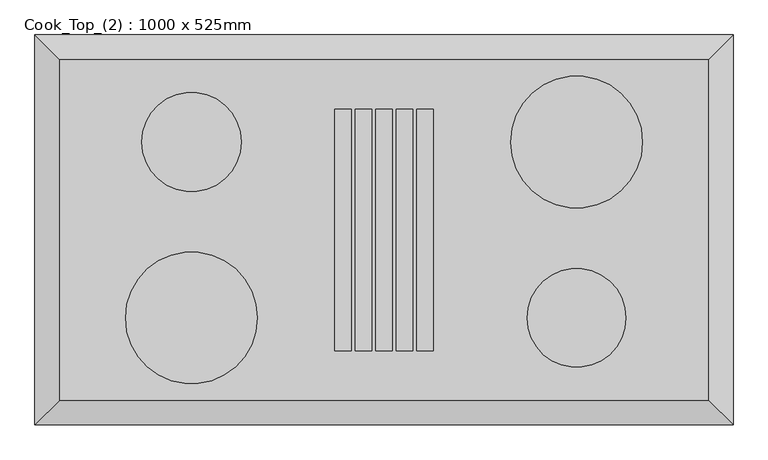
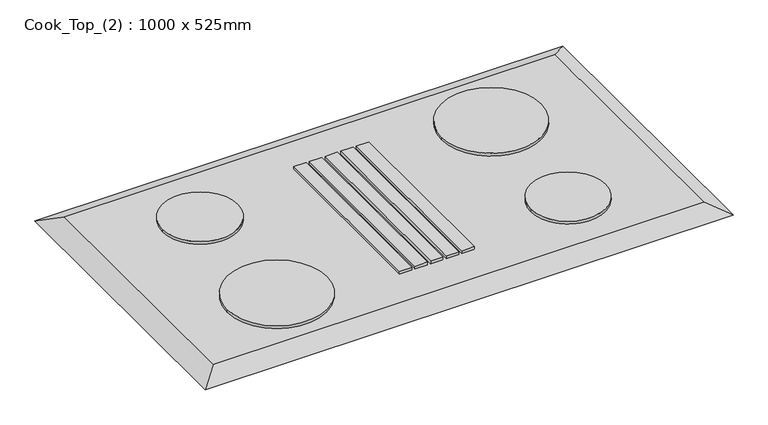
"""IFC4 building model written with IfcOpenShell, lengths in millimetres: proxy geometry, Cook_Top_(2) : 1000 x 525mm."""

from ifc_helpers import new_model, si_unit, point, frame, frame_2d, origin, place, context, project, spatial, polyline, circle_curve, trimmed, segment, composite_curve, outline, extrude, faceted_brep, source, transform, mapped, element, save


def cook_top_2_1000_x_525mm_c9be7e00(model_context):
    return source(origin(), model_context, "Body", "SolidModel", [
        faceted_brep([(500.0, 262.5, 918.0), (-500.0, 262.5, 918.0), (-500.0, -262.5, 918.0), (500.0, -262.5, 918.0), (538.1, 300.6, 900.0), (538.1, -300.6, 900.0), (-538.1, -300.6, 900.0), (-538.1, 300.6, 900.0)], [[[0, 1, 2, 3]], [[4, 5, 6, 7]], [[4, 7, 1, 0]], [[7, 6, 2, 1]], [[6, 5, 3, 2]], [[5, 4, 0, 3]]]),
        extrude(outline(composite_curve([segment(trimmed(circle_curve(frame_2d((-296.8, 135.5)), 76.5869489), [point((-220.2130511, 135.5))], [point((-373.3869489, 135.5))], False, "CARTESIAN"), True, "CONTINUOUS"), segment(trimmed(circle_curve(frame_2d((-296.8, 135.5)), 76.5869489), [point((-373.3869489, 135.5))], [point((-220.2130511, 135.5))], False, "CARTESIAN"), True, "CONTINUOUS")], self_intersect=False)), frame((0.0, 0.0, 918.0), z_axis=(0.0, 0.0, 1.0), x_axis=(1.0, 0.0, 0.0)), (0.0, 0.0, 1.0), 6.35),
        extrude(outline(composite_curve([segment(trimmed(circle_curve(frame_2d((296.8, 135.5)), 101.6), [point((398.4, 135.5))], [point((195.2, 135.5))], False, "CARTESIAN"), True, "CONTINUOUS"), segment(trimmed(circle_curve(frame_2d((296.8, 135.5)), 101.6), [point((195.2, 135.5))], [point((398.4, 135.5))], False, "CARTESIAN"), True, "CONTINUOUS")], self_intersect=False)), frame((0.0, 0.0, 918.0), z_axis=(0.0, 0.0, 1.0), x_axis=(1.0, 0.0, 0.0)), (0.0, 0.0, 1.0), 6.35),
        extrude(outline(composite_curve([segment(trimmed(circle_curve(frame_2d((296.8, -135.5)), 76.2), [point((373.0, -135.5))], [point((220.6, -135.5))], False, "CARTESIAN"), True, "CONTINUOUS"), segment(trimmed(circle_curve(frame_2d((296.8, -135.5)), 76.2), [point((220.6, -135.5))], [point((373.0, -135.5))], False, "CARTESIAN"), True, "CONTINUOUS")], self_intersect=False)), frame((0.0, 0.0, 918.0), z_axis=(0.0, 0.0, 1.0), x_axis=(1.0, 0.0, 0.0)), (0.0, 0.0, 1.0), 6.35),
        extrude(outline(polyline([(-50.8, 186.3), (-50.8, -186.3), (-76.2, -186.3), (-76.2, 186.3), (-50.8, 186.3)])), frame((0.0, 0.0, 918.0), z_axis=(0.0, 0.0, 1.0), x_axis=(1.0, 0.0, 0.0)), (0.0, 0.0, 1.0), 6.35),
        extrude(outline(polyline([(-19.05, 186.3), (-19.05, -186.3), (-44.45, -186.3), (-44.45, 186.3), (-19.05, 186.3)])), frame((0.0, 0.0, 918.0), z_axis=(0.0, 0.0, 1.0), x_axis=(1.0, 0.0, 0.0)), (0.0, 0.0, 1.0), 6.35),
        extrude(outline(polyline([(12.7, 186.3), (12.7, -186.3), (-12.7, -186.3), (-12.7, 186.3), (12.7, 186.3)])), frame((0.0, 0.0, 918.0), z_axis=(0.0, 0.0, 1.0), x_axis=(1.0, 0.0, 0.0)), (0.0, 0.0, 1.0), 6.35),
        extrude(outline(polyline([(44.45, 186.3), (44.45, -186.3), (19.05, -186.3), (19.05, 186.3), (44.45, 186.3)])), frame((0.0, 0.0, 918.0), z_axis=(0.0, 0.0, 1.0), x_axis=(1.0, 0.0, 0.0)), (0.0, 0.0, 1.0), 6.35),
        extrude(outline(polyline([(76.2, 186.3), (76.2, -186.3), (50.8, -186.3), (50.8, 186.3), (76.2, 186.3)])), frame((0.0, 0.0, 918.0), z_axis=(0.0, 0.0, 1.0), x_axis=(1.0, 0.0, 0.0)), (0.0, 0.0, 1.0), 6.35),
        extrude(outline(composite_curve([segment(trimmed(circle_curve(frame_2d((-296.8, -135.5)), 101.6), [point((-195.2, -135.5))], [point((-398.4, -135.5))], False, "CARTESIAN"), True, "CONTINUOUS"), segment(trimmed(circle_curve(frame_2d((-296.8, -135.5)), 101.6), [point((-398.4, -135.5))], [point((-195.2, -135.5))], False, "CARTESIAN"), True, "CONTINUOUS")], self_intersect=False)), frame((0.0, 0.0, 918.0), z_axis=(0.0, 0.0, 1.0), x_axis=(1.0, 0.0, 0.0)), (0.0, 0.0, 1.0), 6.35),
    ])


if __name__ == "__main__":
    model = new_model("IFC4")
    model_context = context("Model", 3, world=origin())
    ifc_project = project(units=[si_unit("LENGTHUNIT", "METRE", prefix="MILLI")], contexts=[model_context])
    site = spatial("IfcSite", under=ifc_project)
    building = spatial("IfcBuilding", under=site)
    placement = place(None, origin())
    cook_top_2_1000_x_525mm_shape = cook_top_2_1000_x_525mm_c9be7e00(model_context)
    element("IfcBuildingElementProxy", 1, Name="Cook_Top_(2) : 1000 x 525mm", ObjectType="Cook_Top_(2) : 1000 x 525mm", at=placement, inside=building, context=model_context, shape_type="MappedRepresentation", body=[
        mapped(cook_top_2_1000_x_525mm_shape, transform((0.0, 0.0, 0.0), x_axis=(1.0, 0.0, 0.0), y_axis=(0.0, 1.0, 0.0), z_axis=(0.0, 0.0, 1.0))),
    ])
    save(model, "model.ifc")

# Revit data of these elements
# Type "Cook_Top_(2) : 1000 x 525mm"
#   Keynote = "N"
#   Depth = 525 mm
#   Width = 1000 mm
#   Material Burner = Metal - Chrome
#   Material Cooktop = Metal - Steel, Polished
#   Default Elevation = 0
# Element 1 (IfcBuildingElementProxy, "Cook_Top_(2) : 1000 x 525mm")
#   Materials on its faces: "Metal - Chrome", "Metal - Steel, Polished"
# Materials
#   "Metal - Chrome": colour RGB 201 201 201, transparency 0
#   "Metal - Steel, Polished": colour RGB 247 247 247, transparency 0
